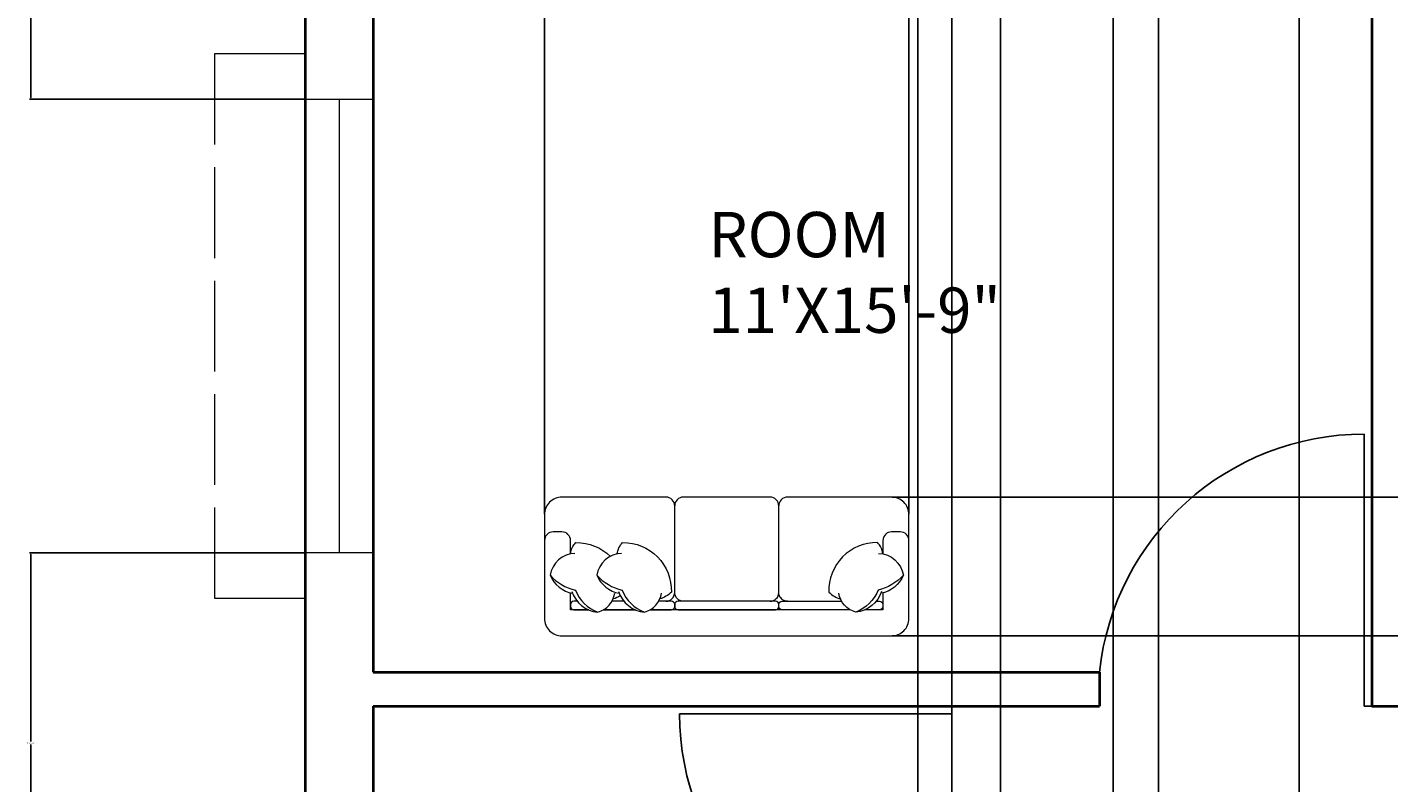
# Model space of a CAD drawing. Units: inches. Extents: x -22 to 362, y -469 to 42.
# Tile 4 of 6: x -22 to 158, y -207 to -107. Entities that reach past the tile are written whole.
import ezdxf

# ---------------------------------------------------------------- set-up
doc = ezdxf.new("R2010")
doc.units = ezdxf.units.IN
doc.header["$MEASUREMENT"] = 0
doc.linetypes.add('ACAD_ISO02W100', pattern=[15, 12, -3])
for name, color, linetype, lineweight in [('A-ANNO-DIMS', 2, 'Continuous', 18), ('A-AREA-IDEN', 7, 'Continuous', 25), ('A-DOOR', 3, 'Continuous', 25), ('A-FURN', 8, 'Continuous', 18), ('A-GLAZ', 4, 'Continuous', 20), ('A-ROOF-OVHD', 8, 'ACAD_ISO02W100', 18), ('A-WALL', 7, 'Continuous', 40)]:
    doc.layers.add(name, color=color, linetype=linetype, lineweight=lineweight)
doc.styles.get("Standard").update_dxf_attribs({"font": 'arial.ttf'})
doc.dimstyles.get("Standard").update_dxf_attribs({"dimtxt": 0.18, "dimasz": 0.18, "dimexe": 0.18, "dimexo": 0.0625, "dimgap": 0.09, "dimtad": 0, "dimtih": 1, "dimtoh": 1, "dimdec": 0, "dimzin": 0, "dimdsep": 46, "dimlunit": 3, "dimtxsty": 'Standard', "dimcen": 0.09, "dimadec": 0, "dimazin": 0, "dimtfac": 1, "dimtdec": 0, "dimtofl": 0, "dimtmove": 0, "dimatfit": 3, "dimfxl": 1, "dimtolj": 1, "dimtzin": 0, "dimarcsym": 0})

# ---------------------------------------------------------------- blocks, each defined once
blk = doc.blocks.new('DOOR-SWING-36')
for p, q in [((-1, 0), (-1, 36)), ((0, 0), (-1, 0))]:
    blk.add_line(p, q)
blk.add_arc((-1, 0.81), 35.19, 90, 173.9744)
blk = doc.blocks.new('WIN-60-WALL9')
for p, q in [((0, 9), (60, 9)), ((0, 0), (0, 9)), ((60, 9), (60, 0)), ((0, 4.5), (60, 4.5)), ((60, 0), (0, 0))]:
    blk.add_line(p, q)
blk = doc.blocks.new('WINDOW-SHADE-72')
for p, q in [((12, 72), (0, 72)), ((12, 0), (12, 72)), ((0, 0), (12, 0))]:
    blk.add_line(p, q)
blk = doc.blocks.new('*D35')
at = {"layer": 'A-ANNO-DIMS', "color": 0, "lineweight": -2, "transparency": 16777216}
for p, q in [((14.95, -78.26), (-21.45, -78.26)), ((-21.27, -78.44), (-21.27, -97.21)), ((-21.27, -116.34), (-21.27, -97.58)), ((14.95, -116.52), (-21.45, -116.52))]:
    blk.add_line(p, q, dxfattribs=at)
at = {"layer": 'A-ANNO-DIMS', "color": 0, "transparency": 16777216}
for points in [[(-21.3, -78.44), (-21.24, -78.44), (-21.27, -78.26)], [(-21.3, -116.34), (-21.24, -116.34), (-21.27, -116.52)]]:
    blk.add_solid(points, dxfattribs=at)
at = {"layer": 'Defpoints', "color": 0, "transparency": 16777216}
for p in [(15.01, -78.26), (-21.27, -116.52), (15.01, -116.52)]:
    blk.add_point(p, dxfattribs=at)
at = {"layer": 'A-ANNO-DIMS', "color": 0, "transparency": 16777216, "insert": (-21.27, -97.39), "char_height": 0.18, "attachment_point": 5}
blk.add_mtext('\\A1;3\'-2 1/2"', dxfattribs=at)
blk = doc.blocks.new('*D36')
at = {"layer": 'A-ANNO-DIMS', "color": 0, "lineweight": -2, "transparency": 16777216}
for p, q in [((14.95, -176.52), (-21.45, -176.52)), ((-21.27, -176.7), (-21.27, -201.48)), ((-21.27, -226.63), (-21.27, -201.85)), ((14.95, -226.81), (-21.45, -226.81))]:
    blk.add_line(p, q, dxfattribs=at)
at = {"layer": 'A-ANNO-DIMS', "color": 0, "transparency": 16777216}
for points in [[(-21.3, -176.7), (-21.24, -176.7), (-21.27, -176.52)], [(-21.3, -226.63), (-21.24, -226.63), (-21.27, -226.81)]]:
    blk.add_solid(points, dxfattribs=at)
at = {"layer": 'Defpoints', "color": 0, "transparency": 16777216}
for p in [(15.01, -176.52), (-21.27, -226.81), (15.01, -226.81)]:
    blk.add_point(p, dxfattribs=at)
at = {"layer": 'A-ANNO-DIMS', "color": 0, "transparency": 16777216, "insert": (-21.27, -201.66), "char_height": 0.18, "attachment_point": 5}
blk.add_mtext('\\A1;4\'-2 1/2"', dxfattribs=at)
blk = doc.blocks.new('*D49')
at = {"layer": 'A-ANNO-DIMS', "color": 0, "lineweight": -2, "transparency": 16777216}
for p, q in [((46.64, -171.38), (46.64, 42.15)), ((46.82, 41.97), (70.4, 41.97)), ((94.64, 41.97), (71.07, 41.97)), ((94.82, -171.38), (94.82, 42.15))]:
    blk.add_line(p, q, dxfattribs=at)
at = {"layer": 'A-ANNO-DIMS', "color": 0, "transparency": 16777216}
for points in [[(46.82, 42), (46.82, 41.94), (46.64, 41.97)], [(94.64, 42), (94.64, 41.94), (94.82, 41.97)]]:
    blk.add_solid(points, dxfattribs=at)
at = {"layer": 'Defpoints', "color": 0, "transparency": 16777216}
for p in [(94.82, 41.97), (46.64, -171.44), (94.82, -171.44)]:
    blk.add_point(p, dxfattribs=at)
at = {"layer": 'A-ANNO-DIMS', "color": 0, "transparency": 16777216, "insert": (70.73, 41.97), "char_height": 0.18, "attachment_point": 5}
blk.add_mtext('\\A1;4\'-0"', dxfattribs=at)
blk = doc.blocks.new('*D50')
at = {"layer": 'A-ANNO-DIMS', "color": 0, "lineweight": -2, "transparency": 16777216}
for p, q in [((92.59, -169.15), (350.97, -169.15)), ((350.79, -169.33), (350.79, -178.14)), ((350.79, -187.32), (350.79, -178.51)), ((92.59, -187.5), (350.97, -187.5))]:
    blk.add_line(p, q, dxfattribs=at)
at = {"layer": 'A-ANNO-DIMS', "color": 0, "transparency": 16777216}
for points in [[(350.76, -169.33), (350.82, -169.33), (350.79, -169.15)], [(350.76, -187.32), (350.82, -187.32), (350.79, -187.5)]]:
    blk.add_solid(points, dxfattribs=at)
at = {"layer": 'Defpoints', "color": 0, "transparency": 16777216}
for p in [(92.53, -169.15), (92.53, -187.5), (350.79, -187.5)]:
    blk.add_point(p, dxfattribs=at)
at = {"layer": 'A-ANNO-DIMS', "color": 0, "transparency": 16777216, "insert": (350.79, -178.33), "char_height": 0.18, "attachment_point": 5}
blk.add_mtext('\\A1;1\'-6 1/2"', dxfattribs=at)
blk = doc.blocks.new('*D51')
at = {"layer": 'A-ANNO-DIMS', "color": 0, "lineweight": -2, "transparency": 16777216}
for p, q in [((96.01, -232.74), (96.01, 42.15)), ((96.19, 41.97), (97.72, 41.97)), ((100.33, 41.97), (98.8, 41.97)), ((100.51, -232.74), (100.51, 42.15))]:
    blk.add_line(p, q, dxfattribs=at)
at = {"layer": 'A-ANNO-DIMS', "color": 0, "transparency": 16777216}
for points in [[(96.19, 42), (96.19, 41.94), (96.01, 41.97)], [(100.33, 42), (100.33, 41.94), (100.51, 41.97)]]:
    blk.add_solid(points, dxfattribs=at)
at = {"layer": 'Defpoints', "color": 0, "transparency": 16777216}
for p in [(100.51, 41.97), (96.01, -232.81), (100.51, -232.81)]:
    blk.add_point(p, dxfattribs=at)
at = {"layer": 'A-ANNO-DIMS', "color": 0, "transparency": 16777216, "insert": (98.26, 41.97), "char_height": 0.18, "attachment_point": 5}
blk.add_mtext('\\A1;0\'-4 1/2"', dxfattribs=at)
blk = doc.blocks.new('*D55')
at = {"layer": 'A-ANNO-DIMS', "color": 0, "lineweight": -2, "transparency": 16777216}
for p, q in [((106.94, -257.14), (106.94, 42.15)), ((107.12, 41.97), (114.06, 41.97)), ((121.63, 41.97), (114.7, 41.97)), ((121.81, -257.14), (121.81, 42.15))]:
    blk.add_line(p, q, dxfattribs=at)
at = {"layer": 'A-ANNO-DIMS', "color": 0, "transparency": 16777216}
for points in [[(107.12, 42), (107.12, 41.94), (106.94, 41.97)], [(121.63, 42), (121.63, 41.94), (121.81, 41.97)]]:
    blk.add_solid(points, dxfattribs=at)
at = {"layer": 'Defpoints', "color": 0, "transparency": 16777216}
for p in [(121.81, 41.97), (106.94, -257.21), (121.81, -257.21)]:
    blk.add_point(p, dxfattribs=at)
at = {"layer": 'A-ANNO-DIMS', "color": 0, "transparency": 16777216, "insert": (114.38, 41.97), "char_height": 0.18, "attachment_point": 5}
blk.add_mtext('\\A1;1\'-3"', dxfattribs=at)
blk = doc.blocks.new('*D56')
at = {"layer": 'A-ANNO-DIMS', "color": 0, "lineweight": -2, "transparency": 16777216}
for p, q in [((127.83, -264.69), (127.83, 42.15)), ((128.01, 41.97), (136.59, 41.97)), ((146.23, 41.97), (137.65, 41.97)), ((146.41, -264.69), (146.41, 42.15))]:
    blk.add_line(p, q, dxfattribs=at)
at = {"layer": 'A-ANNO-DIMS', "color": 0, "transparency": 16777216}
for points in [[(128.01, 42), (128.01, 41.94), (127.83, 41.97)], [(146.23, 42), (146.23, 41.94), (146.41, 41.97)]]:
    blk.add_solid(points, dxfattribs=at)
at = {"layer": 'Defpoints', "color": 0, "transparency": 16777216}
for p in [(146.41, 41.97), (127.83, -264.76), (146.41, -264.76)]:
    blk.add_point(p, dxfattribs=at)
at = {"layer": 'A-ANNO-DIMS', "color": 0, "transparency": 16777216, "insert": (137.12, 41.97), "char_height": 0.18, "attachment_point": 5}
blk.add_mtext('\\A1;1\'-6 1/2"', dxfattribs=at)

msp = doc.modelspace()

# ---------------------------------------------------------------- linework, layer by layer
at = {"layer": 'A-FURN', "ltscale": 0.03}
msp.add_lwpolyline([(94.82, -171.44, 0.414214), (92.53, -169.15), (78.76, -169.15, 0.414214), (77.62, -170.3, 0.414214), (76.47, -169.15), (65, -169.15, 0.414214), (63.85, -170.3, 0.414214), (62.7, -169.15), (48.94, -169.15, 0.414214), (46.64, -171.44), (46.64, -185.21, 0.414214), (48.94, -187.5), (92.53, -187.5, 0.414214), (94.82, -185.21)], format="xyb", close=True, dxfattribs=at)
at = {"layer": 'A-FURN'}
for points in [[(62.7, -182.91, 0.414214), (63.85, -181.77), (63.85, -170.3, 0.414214)], [(78.76, -182.91, -0.414214), (77.62, -181.77), (77.62, -170.3, -0.414214)], [(50.08, -176.66), (50.08, -174.88, 0.414214), (48.94, -173.74), (47.79, -173.74, 0.414214), (46.64, -174.88)], [(94.82, -174.88, 0.414214), (93.68, -173.74), (92.53, -173.74, 0.414214), (91.38, -174.88), (91.38, -176.66)], [(50.08, -176.66, -0.165541), (50.79, -175.15, -0.200231), (55.35, -176.99, -0.121523)], [(56.26, -176.66, -0.165541), (56.97, -175.15, -0.425989), (63.41, -181.72, -0.121523), (61.88, -182.62, 7.115464)], [(91.38, -176.66, 0.165541), (90.67, -175.15, 0.425989), (84.23, -181.72, 0.121523), (85.76, -182.62, -7.115464)], [(50.66, -176.59, 0.356772), (47.37, -179.48, 0.249542), (50.35, -181.87, -9.61688)], [(56.84, -176.59, 0.356772), (53.55, -179.48, 0.249542), (56.53, -181.87, -9.61688)], [(90.81, -176.59, -0.356772), (94.09, -179.48, -0.249542), (91.11, -181.87, 9.61688)], [(47.37, -179.48, 0.14773), (50.73, -181.46, 0.213343), (53.68, -184.35, 0.178662)], [(53.55, -179.48, 0.14773), (56.91, -181.46, 0.213343), (59.86, -184.35, 0.178662)], [(94.09, -179.48, -0.14773), (90.74, -181.46, -0.213343), (87.78, -184.35, -0.178662)], [(52.5, -184.06), (50.08, -184.06), (50.08, -181.81, 0.414214)], [(50.26, -181.61, 0.306663), (53.68, -184.35, 0.30633), (55.92, -181.85, -0.872847)], [(56.44, -181.61, 0.306663), (59.86, -184.35, 0.30633), (62.1, -181.85, -0.872847)], [(65, -182.91, -0.414214), (63.85, -181.77)], [(76.47, -182.91, 0.414214), (77.62, -181.77)], [(91.2, -181.61, -0.306663), (87.78, -184.35, -0.30633), (85.55, -181.85, 0.872847)], [(50.96, -182.91), (50.54, -182.91, 0.414214), (50.08, -183.37), (50.08, -183.6, 0.414214), (50.54, -184.06)], [(57.14, -182.91), (55.56, -182.91, 0.414214)], [(56.67, -182.18, -0.071865), (55.71, -182.62, 7.115464)], [(60.59, -184.06), (63.39, -184.06, 0.414214), (63.85, -183.6), (63.85, -183.37, 0.414214), (63.39, -182.91), (61.74, -182.91, 0.414214)], [(87.06, -184.06), (78.07, -184.06, -0.414214), (77.62, -183.6), (77.62, -183.37, -0.414214), (78.07, -182.91), (85.9, -182.91, -0.414214)], [(90.51, -182.91), (90.92, -182.91, -0.414214), (91.38, -183.37), (91.38, -183.6, -0.414214), (90.92, -184.06)], [(50.54, -184.06), (52.5, -184.06, 0.414214)], [(54.41, -184.06), (58.68, -184.06, 0.414214)], [(90.92, -184.06), (88.97, -184.06, -0.414214)]]:
    msp.add_lwpolyline(points, format="xyb", dxfattribs=at)
for points in [[(91.38, -181.81), (91.38, -184.06), (88.97, -184.06)], [(58.68, -184.06), (54.41, -184.06)], [(87.06, -184.06), (60.59, -184.06)]]:
    msp.add_lwpolyline(points, dxfattribs=at)
msp.add_lwpolyline([(64.31, -184.06), (77.16, -184.06, 0.414214), (77.62, -183.6), (77.62, -183.37, 0.414214), (77.16, -182.91), (64.31, -182.91, 0.414214), (63.85, -183.37), (63.85, -183.6, 0.414214)], format="xyb", close=True, dxfattribs=at)
at = {"layer": 'A-WALL'}
for p, q in [((15.01, 5.69), (15.01, -414.31)), ((24.01, -3.31), (24.01, -192.31)), ((156.01, -3.31), (156.01, -196.81)), ((24.01, -192.31), (120.01, -192.31)), ((120.01, -192.31), (120.01, -196.81)), ((24.01, -196.81), (120.01, -196.81)), ((24.01, -196.81), (24.01, -316.81)), ((156.01, -196.81), (160.51, -196.81))]:
    msp.add_line(p, q, dxfattribs=at)

# ---------------------------------------------------------------- block references
at = {"layer": 'A-DOOR'}
msp.add_blockref('DOOR-SWING-36', (156.01, -196.81), dxfattribs=at)
at = {"layer": 'A-DOOR', "rotation": 90}
msp.add_blockref('DOOR-SWING-36', (100.51, -196.81), dxfattribs=at)
at = {"layer": 'A-GLAZ', "rotation": 270}
msp.add_blockref('WIN-60-WALL9', (15.01, -116.52), dxfattribs=at)
at = {"layer": 'A-ROOF-OVHD', "rotation": 180}
msp.add_blockref('WINDOW-SHADE-72', (15.01, -110.52), dxfattribs=at)

# ---------------------------------------------------------------- texts
at = {"layer": 'A-AREA-IDEN', "insert": (68.3, -131.42), "char_height": 6, "attachment_point": 1}
msp.add_mtext('ROOM\\P11\'X15\'-9"', dxfattribs=at)

# ---------------------------------------------------------------- dimensions: what is measured, and where the dimension line sits
at = {"layer": 'A-ANNO-DIMS'}
for base, p1, p2, picture, middle in [((94.82, 41.97), (46.64, -171.44), (94.82, -171.44), '*D49', (70.73, 41.97)), ((100.51, 41.97), (96.01, -232.81), (100.51, -232.81), '*D51', (98.26, 41.97)), ((121.81, 41.97), (106.94, -257.21), (121.81, -257.21), '*D55', (114.38, 41.97)), ((146.41, 41.97), (127.83, -264.76), (146.41, -264.76), '*D56', (137.12, 41.97))]:
    dim = msp.add_linear_dim(base=base, p1=p1, p2=p2, dimstyle='Standard', override={"dimdec": 1, "dimlfac": 1, "dimrnd": 0, "dimzin": 1, "dimdsep": 46, "dimlunit": 4, "dimfrac": 2}, dxfattribs=at)
    dim.commit()
    dim.dimension.update_dxf_attribs({"geometry": picture, "text_midpoint": middle})
for base, p1, p2, picture, middle in [((-21.27, -116.52), (15.01, -78.26), (15.01, -116.52), '*D35', (-21.27, -97.39)), ((350.7908, -187.5033), (92.5287, -169.1491), (92.5287, -187.5033), '*D50', (350.7908, -178.3262)), ((-21.27, -226.81), (15.01, -176.52), (15.01, -226.81), '*D36', (-21.27, -201.66))]:
    dim = msp.add_linear_dim(base=base, p1=p1, p2=p2, angle=90, dimstyle='Standard', override={"dimdec": 1, "dimlfac": 1, "dimrnd": 0, "dimzin": 1, "dimdsep": 46, "dimlunit": 4, "dimfrac": 2}, dxfattribs=at)
    dim.commit()
    dim.dimension.update_dxf_attribs({"geometry": picture, "text_midpoint": middle})

doc.saveas('drawing.dxf')
